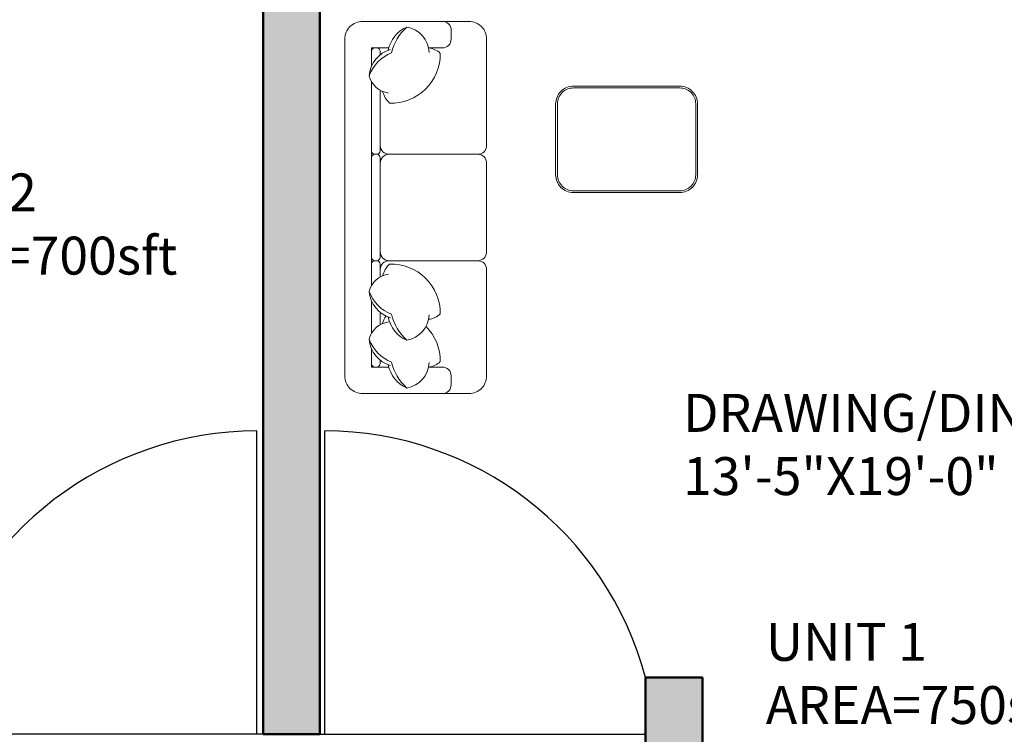
# Model space of a CAD drawing. Units: inches. Extents: x -12 to 604, y -566 to 58.
# Tile 8 of 12: x 280 to 436, y -332 to -219. Entities that reach past the tile are written whole.
import ezdxf

# ---------------------------------------------------------------- set-up
doc = ezdxf.new("R2010")
doc.units = ezdxf.units.IN
doc.header["$MEASUREMENT"] = 0
for name, color, linetype, lineweight in [('A-AREA-IDEN', 7, 'Continuous', 18), ('A-DOOR', 4, 'Continuous', 25), ('A-FURN', 8, 'Continuous', 18), ('A-WALL', 7, 'Continuous', 50), ('A-WALL-PATT', 18, 'Continuous', 13)]:
    doc.layers.add(name, color=color, linetype=linetype, lineweight=lineweight)
doc.styles.get("Standard").update_dxf_attribs({"font": 'arial.ttf'})

# ---------------------------------------------------------------- blocks, each defined once
blk = doc.blocks.new('COFFEE-TABLE')
at = {"ltscale": 0.03}
for points in [[(0, 2.81), (0, 14.03, -0.414214), (2.81, 16.83), (19.64, 16.83, -0.414214), (22.44, 14.03), (22.44, 2.81, -0.414214), (19.64, 0), (2.81, 0, -0.414214)], [(0.28, 2.81), (0.28, 14.03, -0.414214), (2.81, 16.55), (19.64, 16.55, -0.414214), (22.16, 14.03), (22.16, 2.81, -0.414214), (19.64, 0.28), (2.81, 0.28, -0.414214)]]:
    blk.add_lwpolyline(points, format="xyb", close=True, dxfattribs=at)

msp = doc.modelspace()

# ---------------------------------------------------------------- hatches: boundary and pattern name
at = {"layer": 'A-WALL-PATT'}
h = msp.add_hatch(color=256, dxfattribs=at)
h.dxf.hatch_style = 1
h.paths.add_polyline_path([(169.32, 11.14), (169.32, 17.14), (160.32, 17.14), (160.32, 11.14), (118.32, 11.14), (118.32, 6.64), (118.32, 2.14), (127.32, 2.14), (169.32, 2.14)])
h.paths.add_polyline_path([(127.32, -13.61), (118.32, -13.61), (118.32, -29.36), (34.82, -29.36), (24.32, -29.36), (24.32, -38.36), (39.32, -38.36), (118.32, -38.36), (118.32, -126.86), (127.32, -126.86), (127.32, -117.86)])
h.paths.add_polyline_path([(82.32, -92.36), (39.32, -92.36), (39.32, -56.22), (30.32, -56.22), (24.32, -56.22), (24.32, -65.22), (30.32, -65.22), (30.32, -113.36), (24.32, -113.36), (24.32, -122.36), (39.32, -122.36), (39.32, -101.36), (82.32, -101.36), (82.32, -96.86)], flags=17)
h.paths.add_polyline_path([(280.32, 11.14), (238.32, 11.14), (238.32, 17.14), (229.32, 17.14), (229.32, 12.64), (229.32, 11.14), (229.32, 2.14), (271.32, 2.14), (271.32, -117.86), (163.32, -117.86), (163.32, -126.86), (271.32, -126.86), (271.32, -189.86), (280.32, -189.86), (280.32, -180.86)])
h.paths.add_polyline_path([(415.32, 17.14), (406.32, 17.14), (406.32, 11.14), (358.32, 11.14), (358.32, -21.86), (367.32, -21.86), (367.32, 2.14), (415.32, 2.14)], flags=17)
h.paths.add_polyline_path([(484.55, -45.86), (448.32, -45.86), (448.32, 2.14), (448.32, 17.14), (439.32, 17.14), (439.32, 12.64), (439.32, 2.14), (439.32, -45.86), (367.32, -45.86), (358.32, -45.86), (358.32, -54.86), (430.32, -54.86), (430.32, -69.59), (430.32, -180.86), (318.82, -180.86), (318.82, -189.86), (318.82, -331.86), (327.82, -331.86), (327.82, -189.86), (439.32, -189.86), (439.32, -180.86), (439.32, -54.86), (483.5, -54.86), (484.55, -54.86)])
h.paths.add_polyline_path([(529.32, 11.14), (481.32, 11.14), (481.32, 17.14), (472.32, 17.14), (472.32, 12.64), (472.32, 2.14), (520.32, 2.14), (520.32, -21.86), (529.32, -21.86)])
h.paths.add_polyline_path([(598.32, -45.86), (582.42, -45.86), (582.42, -50.36), (582.42, -54.86), (589.32, -54.86), (589.32, -99.86), (598.32, -99.86), (604.32, -99.86), (604.32, -90.86), (598.32, -90.86)])
h.paths.add_polyline_path([(598.32, -168.86), (604.32, -168.86), (604.32, -159.86), (589.32, -159.86), (589.32, -180.86), (477.32, -180.86), (477.32, -189.86), (477.32, -259.86), (486.32, -259.86), (486.32, -189.86), (589.32, -189.86), (589.32, -204.86), (598.32, -204.86), (604.32, -204.86), (604.32, -195.86), (598.32, -195.86)])
h.paths.add_polyline_path([(598.32, -244.86), (604.32, -244.86), (604.32, -235.86), (598.32, -235.86), (589.32, -235.86), (589.32, -250.86), (522.32, -250.86), (522.32, -259.86), (589.32, -259.86), (589.32, -274.86), (598.32, -274.86), (604.32, -274.86), (604.32, -265.86), (598.32, -265.86)])
h.paths.add_polyline_path([(598.32, -333.28), (604.32, -333.28), (604.32, -324.28), (598.32, -324.28), (598.32, -321.87), (598.32, -318.28), (604.32, -318.28), (604.32, -309.28), (598.32, -309.28), (589.32, -309.28), (589.32, -341.95), (589.38, -341.95), (589.38, -363.16), (589.32, -381.86), (565.32, -381.86), (565.32, -390.86), (589.32, -390.86), (589.32, -450.86), (598.32, -450.86), (604.32, -450.86), (604.32, -441.86), (598.32, -441.86), (598.32, -390.86), (604.32, -390.86), (604.32, -381.86), (598.32, -381.86)])
h.paths.add_polyline_path([(541.32, -345.86), (424.32, -345.86), (424.32, -354.86), (532.32, -354.86), (532.32, -474.86), (463.39, -474.86), (463.39, -483.86), (553.32, -483.86), (553.32, -474.86), (541.32, -474.86), (541.32, -390.86), (541.32, -381.86)])
h.paths.add_polyline_path([(604.32, -474.86), (589.32, -474.86), (553.32, -474.86), (553.32, -483.86), (598.32, -483.86), (604.32, -483.86)])
h.paths.add_polyline_path([(388.32, -483.86), (388.32, -474.86), (388.32, -460.13), (388.32, -333.86), (388.32, -322.86), (379.32, -322.86), (379.32, -331.86), (379.32, -333.86), (379.32, -474.86), (379.32, -520.86), (344.32, -520.86), (344.32, -529.86), (379.32, -529.86), (388.32, -529.86)])
h.paths.add_polyline_path([(284.32, -520.86), (249.32, -520.86), (249.32, -474.86), (249.32, -368.36), (240.32, -368.36), (240.32, -474.86), (238.52, -474.86), (238.52, -483.86), (240.32, -483.86), (240.32, -529.86), (249.32, -529.86), (284.32, -529.86)])
h.paths.add_polyline_path([(178.82, -474.86), (158.91, -474.86), (158.91, -483.86), (162.32, -483.86), (178.82, -483.86)])
h.paths.add_polyline_path([(84.32, -474.86), (84.32, -366.86), (75.32, -366.86), (75.32, -474.86), (39.32, -474.86), (39.32, -453.86), (24.32, -453.86), (24.32, -462.86), (30.32, -462.86), (30.32, -483.86), (84.32, -483.86)])
h.paths.add_polyline_path([(39.32, -342.86), (75.32, -342.86), (84.32, -342.86), (179.67, -342.86), (179.67, -333.86), (39.32, -333.86), (39.32, -318.86), (24.32, -318.86), (24.32, -327.86), (30.32, -327.86), (30.32, -432.86), (24.32, -432.86), (24.32, -441.86), (30.32, -441.86), (39.32, -441.86)])
h.paths.add_polyline_path([(249.32, -252.86), (115.32, -252.86), (115.32, -225.86), (106.32, -225.86), (106.32, -252.86), (39.32, -252.86), (39.32, -237.86), (24.32, -237.86), (24.32, -246.86), (30.32, -246.86), (30.32, -267.86), (24.32, -267.86), (24.32, -276.86), (39.32, -276.86), (39.32, -261.86), (240.32, -261.86), (240.32, -331.86), (249.32, -331.86), (266.82, -331.86), (266.82, -322.86), (249.32, -322.86)])
h.paths.add_polyline_path([(127.32, -180.86), (39.32, -180.86), (24.32, -180.86), (24.32, -189.86), (39.32, -189.86), (127.32, -189.86)])
h.paths.add_polyline_path([(39.32, -159.86), (24.32, -159.86), (24.32, -168.86), (30.32, -168.86), (30.32, -180.86), (39.32, -180.86)])
h.paths.add_polyline_path([(470.51, -17.27), (512.48, -17.27), (512.48, 5.12), (470.51, 5.12)], flags=9)
h.paths.add_polyline_path([(484.21, -244.26), (526.45, -244.26), (526.45, -221.87), (484.21, -221.87)], flags=24)
h.paths.add_polyline_path([(36.91, -442.88), (83.54, -442.88), (83.54, -420.5), (36.91, -420.5)], flags=25)

# ---------------------------------------------------------------- linework, layer by layer
at = {"layer": 'A-DOOR'}
for p, q in [((317.86, -295.86), (317.86, -283.86)), ((328.6, -295.86), (328.6, -283.86)), ((317.86, -331.86), (317.86, -295.86)), ((328.6, -331.86), (328.6, -295.86)), ((318.82, -331.86), (266.82, -331.86)), ((327.82, -331.86), (379.32, -331.86))]:
    msp.add_line(p, q, dxfattribs=at)
for centre, radius, start, end in [((317.86, -336.76), 52.9, 90, 164.7673), ((328.6, -336.35), 52.49, 14.8898, 90)]:
    msp.add_arc(centre, radius, start, end, dxfattribs=at)
at = {"layer": 'A-FURN', "ltscale": 0.03}
msp.add_lwpolyline([(351.39, -219.04, -0.414214), (354.19, -221.85), (354.19, -238.68, -0.414214), (352.79, -240.08, -0.414214), (354.19, -241.48), (354.19, -255.51, -0.414214), (352.79, -256.91, -0.414214), (354.19, -258.31), (354.19, -275.14, -0.414214), (351.39, -277.95), (334.56, -277.95, -0.414214), (331.75, -275.14), (331.75, -221.85, -0.414214), (334.56, -219.04)], format="xyb", close=True, dxfattribs=at)
at = {"layer": 'A-FURN'}
for points in [[(347.18, -219.04, -0.414214), (348.58, -220.45), (348.58, -221.85, -0.414214), (347.18, -223.25), (345.01, -223.25)], [(341.56, -219.94, 0.14773), (339.15, -224.03, 0.213343), (335.61, -227.65, 0.178662)], [(345.09, -223.95, 0.356772), (341.56, -219.94, 0.249542), (338.64, -223.58, -9.61688)], [(338.96, -223.47, 0.306663), (335.61, -227.65, 0.30633), (338.67, -230.38, -0.872847)], [(337.36, -224.32), (337.36, -223.81, 0.414214), (336.8, -223.25), (336.52, -223.25, 0.414214), (335.96, -223.81)], [(335.96, -223.81), (335.96, -226.2, 0.414214)], [(345.01, -223.25, -0.165541), (346.86, -224.11, -0.425989), (338.83, -231.99, -0.121523), (337.72, -230.12, 7.115464)], [(335.96, -228.53), (335.96, -239.52, 0.414214), (336.52, -240.08), (336.8, -240.08, 0.414214), (337.36, -239.52), (337.36, -229.95, 0.414214)], [(337.36, -238.68, 0.414214), (338.77, -240.08), (352.79, -240.08, 0.414214)], [(337.36, -241.48, -0.414214), (338.77, -240.08)], [(335.96, -260.9), (335.96, -257.47, -0.414214), (336.52, -256.91), (336.8, -256.91, -0.414214), (337.36, -257.47), (337.36, -259.49, -0.414214)], [(337.36, -255.51, 0.414214), (338.77, -256.91)], [(337.36, -258.31, -0.414214), (338.77, -256.91), (352.79, -256.91, -0.414214)], [(345.01, -266.19, 0.165541), (346.86, -265.32, 0.425989), (338.83, -257.44, 0.121523), (337.72, -259.31, -7.115464)], [(338.96, -265.97, -0.306663), (335.61, -261.78, -0.30633), (338.67, -259.05, 0.872847)], [(341.56, -269.5, -0.14773), (339.15, -265.4, -0.213343), (335.61, -261.78, -0.178662)], [(335.96, -268.46), (335.96, -263.24, -0.414214)], [(337.36, -265.12), (337.36, -267.04, -0.414214)], [(338.27, -265.69, 0.071865), (337.72, -266.87, -7.115464)], [(345.09, -265.48, -0.356772), (341.56, -269.5, -0.249542), (338.64, -265.86, 9.61688)], [(338.96, -273.52, -0.306663), (335.61, -269.34, -0.30633), (338.67, -266.61, 0.872847)], [(345.01, -273.74, 0.165541), (346.86, -272.88, 0.200231), (344.6, -267.31, 0.121523)], [(341.56, -277.06, -0.14773), (339.15, -272.96, -0.213343), (335.61, -269.34, -0.178662)], [(335.96, -270.79), (335.96, -273.74), (338.72, -273.74, -0.414214)], [(335.96, -273.18), (335.96, -270.79, -0.414214)], [(337.36, -272.67), (337.36, -273.18, -0.414214), (336.8, -273.74), (336.52, -273.74, -0.414214), (335.96, -273.18)], [(345.09, -273.04, -0.356772), (341.56, -277.06, -0.249542), (338.64, -273.41, 9.61688)], [(345.01, -273.74), (347.18, -273.74, -0.414214), (348.58, -275.14), (348.58, -276.55, -0.414214), (347.18, -277.95)]]:
    msp.add_lwpolyline(points, format="xyb", dxfattribs=at)
for points in [[(338.72, -223.25), (335.96, -223.25), (335.96, -226.2)], [(335.96, -228.53), (335.96, -260.9)], [(335.96, -263.24), (335.96, -268.46)]]:
    msp.add_lwpolyline(points, dxfattribs=at)
msp.add_lwpolyline([(335.96, -256.35), (335.96, -240.64, -0.414214), (336.52, -240.08), (336.8, -240.08, -0.414214), (337.36, -240.64), (337.36, -256.35, -0.414214), (336.8, -256.91), (336.52, -256.91, -0.414214)], format="xyb", close=True, dxfattribs=at)
at = {"layer": 'A-WALL'}
for p, q in [((318.82, -180.86), (318.82, -331.86)), ((327.82, -189.86), (327.82, -331.86)), ((379.32, -322.86), (388.32, -322.86)), ((379.32, -331.86), (379.32, -322.86)), ((388.32, -322.86), (388.32, -333.86)), ((318.82, -331.86), (327.82, -331.86)), ((379.32, -331.86), (379.32, -333.86))]:
    msp.add_line(p, q, dxfattribs=at)

# ---------------------------------------------------------------- block references
at = {"layer": 'A-FURN'}
msp.add_blockref('COFFEE-TABLE', (365.11, -246.13), dxfattribs=at)

# ---------------------------------------------------------------- texts
at = {"layer": 'A-AREA-IDEN', "char_height": 6, "attachment_point": 1}
for s, insert in [('UNIT 2\\PAREA=700sft', (257.54, -243.11)), ('DRAWING/DINING\\P13\'-5"X19\'-0"', (385.25, -278)), ('UNIT 1\\PAREA=750sft', (398.35, -314.23))]:
    msp.add_mtext(s, dxfattribs=dict(at, insert=insert))

doc.saveas('drawing.dxf')
